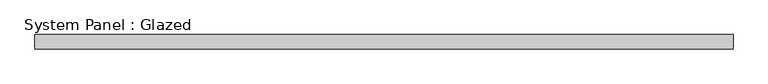
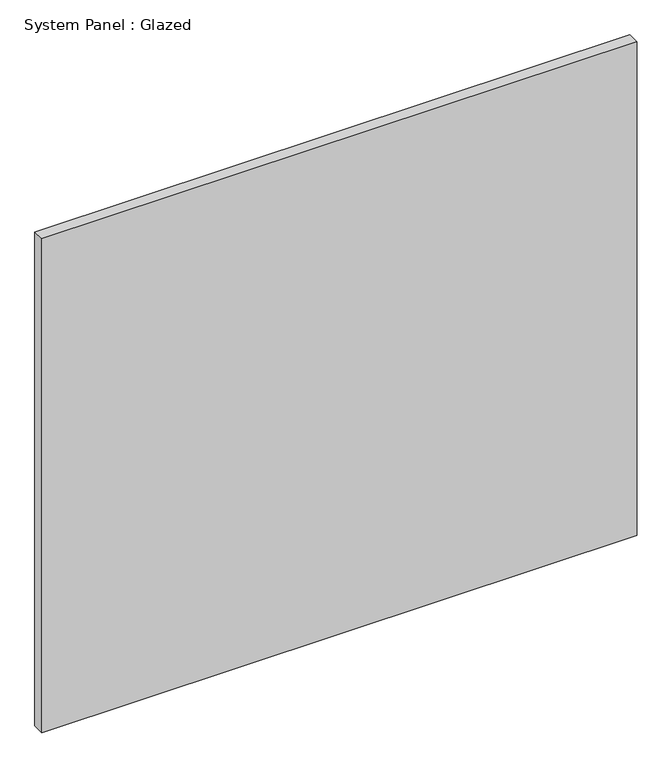
"""IFC4 building model written with IfcOpenShell, lengths in millimetres: plate geometry, System Panel : Glazed."""

from ifc_helpers import new_model, si_unit, origin, origin_with_axes, place, context, project, spatial, polyline, outline, extrude, source, transform, mapped, element, save


def system_panel_glazed_53e0be6b(model_context):
    return source(origin(), model_context, "Body", "SweptSolid", [
        extrude(outline(polyline([(622.3, 19.05), (-622.3, 19.05), (-622.3, 44.45), (622.3, 44.45), (622.3, 19.05)])), origin_with_axes(), (0.0, 0.0, 1.0), 1092.2),
    ])


if __name__ == "__main__":
    model = new_model("IFC4")
    model_context = context("Model", 3, world=origin())
    ifc_project = project(units=[si_unit("LENGTHUNIT", "METRE", prefix="MILLI")], contexts=[model_context])
    site = spatial("IfcSite", under=ifc_project)
    building = spatial("IfcBuilding", under=site)
    placement = place(None, origin())
    system_panel_glazed_shape = system_panel_glazed_53e0be6b(model_context)
    element("IfcPlate", 1, ObjectType="System Panel : Glazed", at=placement, inside=building, context=model_context, shape_type="MappedRepresentation", body=[
        mapped(system_panel_glazed_shape, transform((0.0, 0.0, 0.0), x_axis=(1.0, 0.0, 0.0), y_axis=(0.0, 1.0, 0.0), z_axis=(0.0, 0.0, 1.0))),
    ])
    save(model, "model.ifc")

# Revit data of these elements
# Type "System Panel : Glazed"
#   Construction Type Id = "GSP4R"
#   Analytic Construction = "1/8 in Pilkington single glazing"
#   Visual Light Transmittance = 0.9
#   Solar Heat Gain Coefficient = 0.86
#   Heat Transfer Coefficient (U) = 1.18115 BTU/(h·ft²·°F)
# Element 1 (IfcPlate, "System Panel : Glazed")
#   Materials on its faces: "Glass"
# Materials
#   "Glass": class "Glass", colour RGB 0 128 192, transparency 0.75, Description = "Soda Lime Glass", Cost = 0
